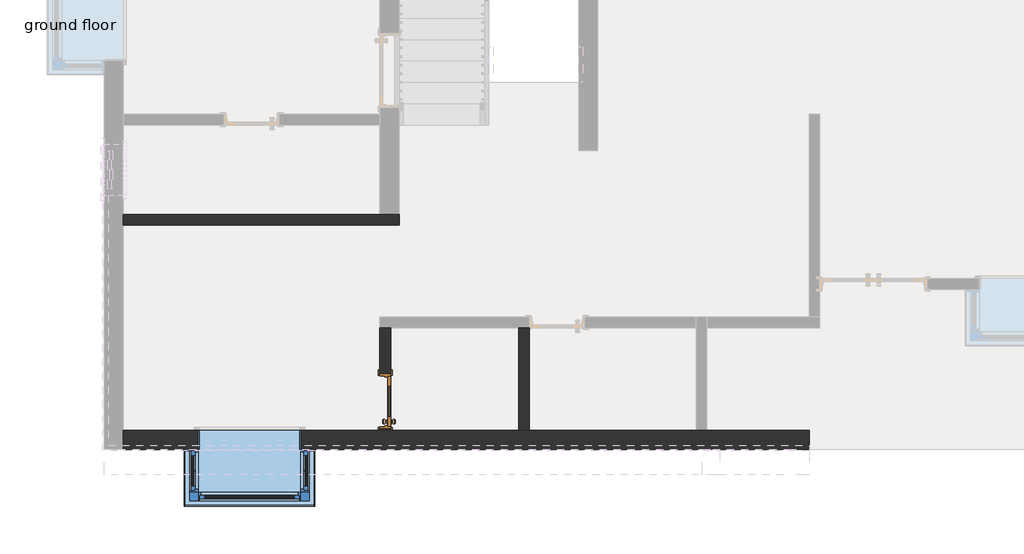
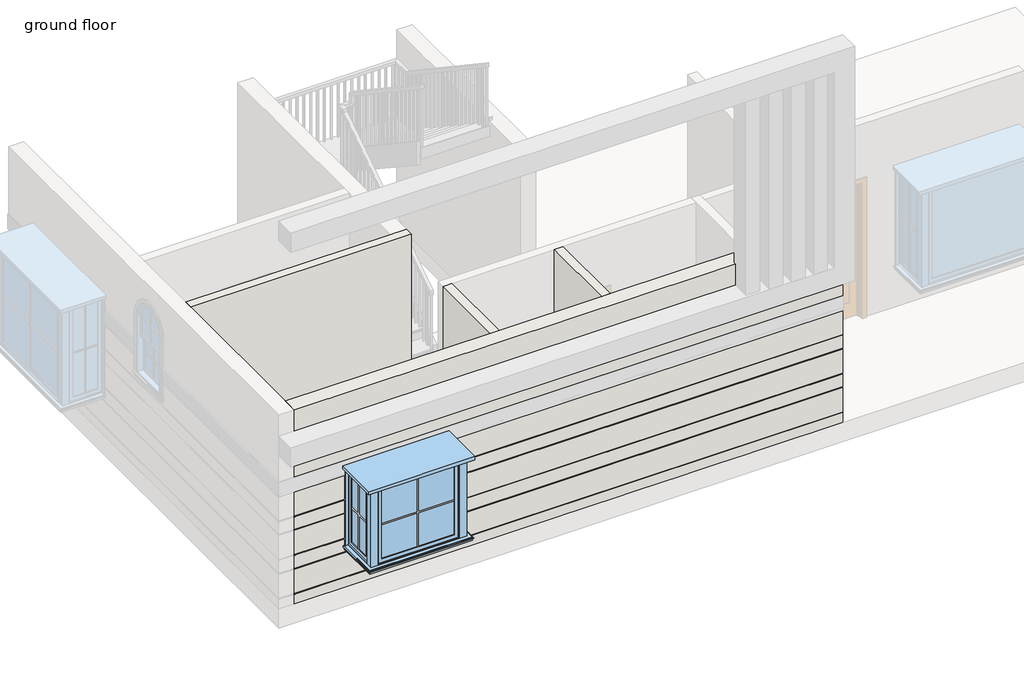
# One storey, part 1 of 5: 4 walls, 1 door, 1 window.
"""IFC4 building model written with IfcOpenShell, lengths in millimetres."""

from ifc_helpers import new_model, si_unit, frame, origin, place, context, project, spatial, polyline, circle_curve, outline, extrude, faceted_brep, transform, mapped, element, save
from ifc_brep_helpers import plane_surface, cylinder_surface, revolved_surface, advanced_brep
from components import door_e337afa5, window_4fde904e

model = new_model("IFC4")

# Units and contexts
model_context = context("Model", 3, world=origin())
ifc_project = project(units=[si_unit("LENGTHUNIT", "METRE", prefix="MILLI")], contexts=[model_context])

# Site, building, storey
site = spatial("IfcSite", under=ifc_project)
building = spatial("IfcBuilding", under=site)
storey = spatial("IfcBuildingStorey", under=building, Name="ground floor", Elevation=304.8)

# Door
placement = place(None, origin())
door_shape = door_e337afa5(model_context)
element("IfcDoor", 1, ObjectType="Door-Interior-Single-2_Panel-Wood : 24\" x 84\"", at=placement, inside=storey, context=model_context, shape_type="MappedRepresentation", body=[
    mapped(door_shape, transform((-9835.7922301, -6693.7302427, 304.8), x_axis=(0.0, 1.0, 0.0), y_axis=(-1.0, 0.0, 0.0), z_axis=(0.0, 0.0, 1.0))),
])

# Walls
element("IfcWall", 2, ObjectType="INNER WALL 5\"", at=placement, inside=storey, context=model_context, shape_type="Brep", body=[
    faceted_brep([(-12950.4672301, -4598.2302427, 304.8), (-9673.8672301, -4598.2302427, 304.8), (-9673.8672301, -4598.2302427, 3352.8), (-12950.4672301, -4598.2302427, 3352.8), (-12950.4672301, -4471.2302427, 304.8), (-12950.4672301, -4471.2302427, 3352.8), (-9902.4672301, -4471.2302427, 3352.8), (-9673.8672301, -4471.2302427, 3352.8), (-9673.8672301, -4471.2302427, 304.8), (-9902.4672301, -4471.2302427, 304.8)], [[[0, 1, 2, 3]], [[4, 5, 6, 7, 8, 9]], [[1, 0, 4, 9, 8]], [[3, 2, 7, 6, 5]], [[0, 3, 5, 4]], [[2, 1, 8, 7]]]),
])
element("IfcWall", 3, ObjectType="INNER WALL 5\"", at=placement, inside=storey, context=model_context, shape_type="Brep", body=[
    faceted_brep([(-8124.4672301, -7036.6302427, 304.8), (-8124.4672301, -5817.4302427, 304.8), (-8124.4672301, -5817.4302427, 2463.8), (-8124.4672301, -5817.4302427, 3352.8), (-8124.4672301, -7036.6302427, 3352.8), (-8251.4672301, -7036.6302427, 304.8), (-8251.4672301, -7036.6302427, 3352.8), (-8251.4672301, -5817.4302427, 3352.8), (-8251.4672301, -5817.4302427, 304.8)], [[[0, 1, 2, 3, 4]], [[5, 6, 7, 8]], [[1, 0, 5, 8]], [[4, 3, 7, 6]], [[0, 4, 6, 5]], [[3, 2, 1, 8, 7]]]),
])
element("IfcWall", 4, ObjectType="INNER WALL 5\"", at=placement, inside=storey, context=model_context, shape_type="SweptSolid", body=[
    extrude(outline(polyline([(-7036.6302427, 3352.8), (-5817.4302427, 3352.8), (-5817.4302427, 304.8), (-6363.5302427, 304.8), (-6363.5302427, 2463.8), (-7023.9302427, 2463.8), (-7023.9302427, 304.8), (-7036.6302427, 304.8), (-7036.6302427, 3352.8)])), frame((-9902.4672301, 0.0, 0.0), z_axis=(1.0, 0.0, 0.0), x_axis=(0.0, 1.0, 0.0)), (0.0, 0.0, 1.0), 127.0),
])
element("IfcWall", 5, ObjectType="OUTER WALL 9\"", at=placement, inside=storey, context=model_context, shape_type="AdvancedBrep", body=[
    advanced_brep(
    [(-12950.4672301, -7265.2302427, 304.8), (-4797.0672301, -7265.2302427, 304.8), (-4797.0672301, -7265.2302427, 455.95311), (-12950.4672301, -7265.2302427, 455.95311), (-4797.0672301, -7265.2302427, 3352.8), (-12950.4672301, -7265.2302427, 3352.8), (-12950.4672301, -7265.2302427, 2298.7), (-4797.0672301, -7265.2302427, 2298.7), (-10842.2672301, -7265.2302427, 914.4), (-12061.4672301, -7265.2302427, 914.4), (-12061.4672301, -7265.2302427, 1065.55311), (-12950.4672301, -7265.2302427, 1065.55311), (-12950.4672301, -7265.2302427, 864.84689), (-12061.4672301, -7265.2302427, 864.84689), (-12061.4672301, -7265.2302427, 850.9), (-12950.4672301, -7265.2302427, 850.9), (-12950.4672301, -7265.2302427, 469.9), (-4797.0672301, -7265.2302427, 469.9), (-4797.0672301, -7265.2302427, 850.9), (-10842.2672301, -7265.2302427, 850.9), (-10842.2672301, -7265.2302427, 864.84689), (-4797.0672301, -7265.2302427, 864.84689), (-4797.0672301, -7265.2302427, 1065.55311), (-10842.2672301, -7265.2302427, 1065.55311), (-12061.4672301, -7265.2302427, 2184.4), (-10842.2672301, -7265.2302427, 2184.4), (-10842.2672301, -7265.2302427, 2084.04689), (-4797.0672301, -7265.2302427, 2084.04689), (-4797.0672301, -7265.2302427, 2284.75311), (-12950.4672301, -7265.2302427, 2284.75311), (-12950.4672301, -7265.2302427, 2084.04689), (-12061.4672301, -7265.2302427, 2084.04689), (-10842.2672301, -7265.2302427, 2070.1), (-10842.2672301, -7265.2302427, 1689.1), (-4797.0672301, -7265.2302427, 1689.1), (-4797.0672301, -7265.2302427, 2070.1), (-10842.2672301, -7265.2302427, 1675.15311), (-10842.2672301, -7265.2302427, 1474.44689), (-4797.0672301, -7265.2302427, 1474.44689), (-4797.0672301, -7265.2302427, 1675.15311), (-12061.4672301, -7265.2302427, 1474.44689), (-12061.4672301, -7265.2302427, 1675.15311), (-12950.4672301, -7265.2302427, 1675.15311), (-12950.4672301, -7265.2302427, 1474.44689), (-4797.0672301, -7265.2302427, 1460.5), (-10842.2672301, -7265.2302427, 1460.5), (-10842.2672301, -7265.2302427, 1079.5), (-4797.0672301, -7265.2302427, 1079.5), (-12061.4672301, -7265.2302427, 2070.1), (-12950.4672301, -7265.2302427, 2070.1), (-12950.4672301, -7265.2302427, 1689.1), (-12061.4672301, -7265.2302427, 1689.1), (-12061.4672301, -7265.2302427, 1460.5), (-12950.4672301, -7265.2302427, 1460.5), (-12950.4672301, -7265.2302427, 1079.5), (-12061.4672301, -7265.2302427, 1079.5), (-4797.0672301, -7036.6302427, 304.8), (-6016.2672301, -7036.6302427, 304.8), (-6143.2672301, -7036.6302427, 304.8), (-8124.4672301, -7036.6302427, 304.8), (-8251.4672301, -7036.6302427, 304.8), (-9775.4672301, -7036.6302427, 304.8), (-9902.4672301, -7036.6302427, 304.8), (-12950.4672301, -7036.6302427, 304.8), (-12950.4672301, -7036.6302427, 3352.8), (-9902.4672301, -7036.6302427, 3352.8), (-9775.4672301, -7036.6302427, 3352.8), (-8251.4672301, -7036.6302427, 3352.8), (-8124.4672301, -7036.6302427, 3352.8), (-6143.2672301, -7036.6302427, 3352.8), (-6016.2672301, -7036.6302427, 3352.8), (-4797.0672301, -7036.6302427, 3352.8), (-12061.4672301, -7036.6302427, 2184.4), (-12061.4672301, -7036.6302427, 914.4), (-10842.2672301, -7036.6302427, 914.4), (-10842.2672301, -7036.6302427, 2184.4), (-4797.0672301, -7216.8686427, 2298.7), (-4797.0672301, -7216.8686427, 2297.3203242), (-4797.0672301, -7221.2514519, 2292.1465897), (-4797.0672301, -7264.1100243, 2285.00348), (-4797.0672301, -7264.1100243, 2083.79652), (-4797.0672301, -7221.2514519, 2076.6534103), (-4797.0672301, -7216.8686427, 2071.4796758), (-4797.0672301, -7216.8686427, 2070.1), (-4797.0672301, -7216.8686427, 1689.1), (-4797.0672301, -7216.8686427, 1687.7203242), (-4797.0672301, -7221.2514519, 1682.5465897), (-4797.0672301, -7264.1100243, 1675.40348), (-4797.0672301, -7264.1100243, 1474.19652), (-4797.0672301, -7221.2514519, 1467.0534103), (-4797.0672301, -7216.8686427, 1461.8796758), (-4797.0672301, -7216.8686427, 1460.5), (-4797.0672301, -7216.8686427, 1079.5), (-4797.0672301, -7216.8686427, 1078.1203242), (-4797.0672301, -7221.2514519, 1072.9465897), (-4797.0672301, -7264.1100243, 1065.80348), (-4797.0672301, -7264.1100243, 864.59652), (-4797.0672301, -7221.2514519, 857.4534103), (-4797.0672301, -7216.8686427, 852.2796758), (-4797.0672301, -7216.8686427, 850.9), (-4797.0672301, -7216.8686427, 469.9), (-4797.0672301, -7216.8686427, 468.5203242), (-4797.0672301, -7221.2514519, 463.3465897), (-4797.0672301, -7264.1100243, 456.20348), (-12950.4672301, -7264.1100243, 456.20348), (-12950.4672301, -7221.2514519, 463.3465897), (-12950.4672301, -7216.8686427, 468.5203242), (-12950.4672301, -7216.8686427, 469.9), (-12950.4672301, -7216.8686427, 850.9), (-12950.4672301, -7216.8686427, 852.2796758), (-12950.4672301, -7221.2514519, 857.4534103), (-12950.4672301, -7264.1100243, 864.59652), (-12950.4672301, -7264.1100243, 1065.80348), (-12950.4672301, -7221.2514519, 1072.9465897), (-12950.4672301, -7216.8686427, 1078.1203242), (-12950.4672301, -7216.8686427, 1079.5), (-12950.4672301, -7216.8686427, 1460.5), (-12950.4672301, -7216.8686427, 1461.8796758), (-12950.4672301, -7221.2514519, 1467.0534103), (-12950.4672301, -7264.1100243, 1474.19652), (-12950.4672301, -7264.1100243, 1675.40348), (-12950.4672301, -7221.2514519, 1682.5465897), (-12950.4672301, -7216.8686427, 1687.7203242), (-12950.4672301, -7216.8686427, 1689.1), (-12950.4672301, -7216.8686427, 2070.1), (-12950.4672301, -7216.8686427, 2071.4796758), (-12950.4672301, -7221.2514519, 2076.6534103), (-12950.4672301, -7264.1100243, 2083.79652), (-12950.4672301, -7264.1100243, 2285.00348), (-12950.4672301, -7221.2514519, 2292.1465897), (-12950.4672301, -7216.8686427, 2297.3203242), (-12950.4672301, -7216.8686427, 2298.7), (-12061.4672301, -7264.1100243, 2083.79652), (-12061.4672301, -7221.2514519, 2076.6534103), (-12061.4672301, -7216.8686427, 2071.4796758), (-12061.4672301, -7216.8686427, 2070.1), (-12061.4672301, -7216.8686427, 1689.1), (-12061.4672301, -7216.8686427, 1687.7203242), (-12061.4672301, -7221.2514519, 1682.5465897), (-12061.4672301, -7264.1100243, 1675.40348), (-12061.4672301, -7264.1100243, 1474.19652), (-12061.4672301, -7221.2514519, 1467.0534103), (-12061.4672301, -7216.8686427, 1461.8796758), (-12061.4672301, -7216.8686427, 1460.5), (-12061.4672301, -7216.8686427, 1079.5), (-12061.4672301, -7216.8686427, 1078.1203242), (-12061.4672301, -7221.2514519, 1072.9465897), (-12061.4672301, -7264.1100243, 1065.80348), (-10842.2672301, -7264.1100243, 1065.80348), (-10842.2672301, -7221.2514519, 1072.9465897), (-10842.2672301, -7216.8686427, 1078.1203242), (-10842.2672301, -7216.8686427, 1079.5), (-10842.2672301, -7216.8686427, 1460.5), (-10842.2672301, -7216.8686427, 1461.8796758), (-10842.2672301, -7221.2514519, 1467.0534103), (-10842.2672301, -7264.1100243, 1474.19652), (-10842.2672301, -7264.1100243, 1675.40348), (-10842.2672301, -7221.2514519, 1682.5465897), (-10842.2672301, -7216.8686427, 1687.7203242), (-10842.2672301, -7216.8686427, 1689.1), (-10842.2672301, -7216.8686427, 2070.1), (-10842.2672301, -7216.8686427, 2071.4796758), (-10842.2672301, -7221.2514519, 2076.6534103), (-10842.2672301, -7264.1100243, 2083.79652), (-10842.2672301, -7221.2514519, 857.4534103), (-10842.2672301, -7264.1100243, 864.59652), (-10842.2672301, -7216.8686427, 850.9), (-10842.2672301, -7216.8686427, 852.2796758), (-12061.4672301, -7216.8686427, 852.2796758), (-12061.4672301, -7216.8686427, 850.9), (-12061.4672301, -7264.1100243, 864.59652), (-12061.4672301, -7221.2514519, 857.4534103)],
    [
        (0, 1),
        (1, 2),
        (2, 3),
        (3, 0),
        (4, 5),
        (5, 6),
        (6, 7),
        (7, 4),
        (8, 9),
        (9, 10),
        (10, 11),
        (11, 12),
        (12, 13),
        (13, 14),
        (14, 15),
        (15, 16),
        (16, 17),
        (17, 18),
        (18, 19),
        (19, 20),
        (20, 21),
        (21, 22),
        (22, 23),
        (23, 8),
        (24, 25),
        (25, 26),
        (26, 27),
        (27, 28),
        (28, 29),
        (29, 30),
        (30, 31),
        (31, 24),
        (32, 33),
        (33, 34),
        (34, 35),
        (35, 32),
        (36, 37),
        (37, 38),
        (38, 39),
        (39, 36),
        (40, 41),
        (41, 42),
        (42, 43),
        (43, 40),
        (44, 45),
        (45, 46),
        (46, 47),
        (47, 44),
        (48, 49),
        (49, 50),
        (50, 51),
        (51, 48),
        (52, 53),
        (53, 54),
        (54, 55),
        (55, 52),
        (56, 57),
        (57, 58),
        (58, 59),
        (59, 60),
        (60, 61),
        (61, 62),
        (62, 63),
        (63, 64),
        (64, 65),
        (65, 66),
        (66, 67),
        (67, 68),
        (68, 69),
        (69, 70),
        (70, 71),
        (71, 56),
        (72, 73),
        (73, 74),
        (74, 75),
        (75, 72),
        (0, 63),
        (56, 1),
        (71, 4),
        (7, 76),
        (76, 77),
        (77, 78, circle_curve(frame((-4797.0672301, -7222.1137427, 2297.3203242), z_axis=(-1.0, 0.0, 0.0), x_axis=(0.0, 1.0, 0.0)), 5.2451)),
        (78, 79),
        (79, 28, circle_curve(frame((-4797.0672301, -7262.3854427, 2274.656011), z_axis=(1.0, 0.0, 0.0), x_axis=(0.0, 1.0, 0.0)), 10.4902)),
        (27, 80, circle_curve(frame((-4797.0672301, -7262.3854427, 2094.143989), z_axis=(1.0, 0.0, 0.0), x_axis=(0.0, 1.0, 0.0)), 10.4902)),
        (80, 81),
        (81, 82, circle_curve(frame((-4797.0672301, -7222.1137427, 2071.4796758), z_axis=(-1.0, 0.0, 0.0), x_axis=(0.0, 1.0, 0.0)), 5.2451)),
        (82, 83),
        (83, 35),
        (34, 84),
        (84, 85),
        (85, 86, circle_curve(frame((-4797.0672301, -7222.1137427, 1687.7203242), z_axis=(-1.0, 0.0, 0.0), x_axis=(0.0, 1.0, 0.0)), 5.2451)),
        (86, 87),
        (87, 39, circle_curve(frame((-4797.0672301, -7262.3854427, 1665.056011), z_axis=(1.0, 0.0, 0.0), x_axis=(0.0, 1.0, 0.0)), 10.4902)),
        (38, 88, circle_curve(frame((-4797.0672301, -7262.3854427, 1484.543989), z_axis=(1.0, 0.0, 0.0), x_axis=(0.0, 1.0, 0.0)), 10.4902)),
        (88, 89),
        (89, 90, circle_curve(frame((-4797.0672301, -7222.1137427, 1461.8796758), z_axis=(-1.0, 0.0, 0.0), x_axis=(0.0, 1.0, 0.0)), 5.2451)),
        (90, 91),
        (91, 44),
        (47, 92),
        (92, 93),
        (93, 94, circle_curve(frame((-4797.0672301, -7222.1137427, 1078.1203242), z_axis=(-1.0, 0.0, 0.0), x_axis=(0.0, 1.0, 0.0)), 5.2451)),
        (94, 95),
        (95, 22, circle_curve(frame((-4797.0672301, -7262.3854427, 1055.456011), z_axis=(1.0, 0.0, 0.0), x_axis=(0.0, 1.0, 0.0)), 10.4902)),
        (21, 96, circle_curve(frame((-4797.0672301, -7262.3854427, 874.943989), z_axis=(1.0, 0.0, 0.0), x_axis=(0.0, 1.0, 0.0)), 10.4902)),
        (96, 97),
        (97, 98, circle_curve(frame((-4797.0672301, -7222.1137427, 852.2796758), z_axis=(-1.0, 0.0, 0.0), x_axis=(0.0, 1.0, 0.0)), 5.2451)),
        (98, 99),
        (99, 18),
        (17, 100),
        (100, 101),
        (101, 102, circle_curve(frame((-4797.0672301, -7222.1137427, 468.5203242), z_axis=(-1.0, 0.0, 0.0), x_axis=(0.0, 1.0, 0.0)), 5.2451)),
        (102, 103),
        (103, 2, circle_curve(frame((-4797.0672301, -7262.3854427, 445.856011), z_axis=(1.0, 0.0, 0.0), x_axis=(0.0, 1.0, 0.0)), 10.4902)),
        (64, 5),
        (3, 104, circle_curve(frame((-12950.4672301, -7262.3854427, 445.856011), z_axis=(-1.0, 0.0, 0.0), x_axis=(0.0, 1.0, 0.0)), 10.4902)),
        (104, 105),
        (105, 106, circle_curve(frame((-12950.4672301, -7222.1137427, 468.5203242), z_axis=(1.0, 0.0, 0.0), x_axis=(0.0, 1.0, 0.0)), 5.2451)),
        (106, 107),
        (107, 16),
        (15, 108),
        (108, 109),
        (109, 110, circle_curve(frame((-12950.4672301, -7222.1137427, 852.2796758), z_axis=(1.0, 0.0, 0.0), x_axis=(0.0, 1.0, 0.0)), 5.2451)),
        (110, 111),
        (111, 12, circle_curve(frame((-12950.4672301, -7262.3854427, 874.943989), z_axis=(-1.0, 0.0, 0.0), x_axis=(0.0, 1.0, 0.0)), 10.4902)),
        (11, 112, circle_curve(frame((-12950.4672301, -7262.3854427, 1055.456011), z_axis=(-1.0, 0.0, 0.0), x_axis=(0.0, 1.0, 0.0)), 10.4902)),
        (112, 113),
        (113, 114, circle_curve(frame((-12950.4672301, -7222.1137427, 1078.1203242), z_axis=(1.0, 0.0, 0.0), x_axis=(0.0, 1.0, 0.0)), 5.2451)),
        (114, 115),
        (115, 54),
        (53, 116),
        (116, 117),
        (117, 118, circle_curve(frame((-12950.4672301, -7222.1137427, 1461.8796758), z_axis=(1.0, 0.0, 0.0), x_axis=(0.0, 1.0, 0.0)), 5.2451)),
        (118, 119),
        (119, 43, circle_curve(frame((-12950.4672301, -7262.3854427, 1484.543989), z_axis=(-1.0, 0.0, 0.0), x_axis=(0.0, 1.0, 0.0)), 10.4902)),
        (42, 120, circle_curve(frame((-12950.4672301, -7262.3854427, 1665.056011), z_axis=(-1.0, 0.0, 0.0), x_axis=(0.0, 1.0, 0.0)), 10.4902)),
        (120, 121),
        (121, 122, circle_curve(frame((-12950.4672301, -7222.1137427, 1687.7203242), z_axis=(1.0, 0.0, 0.0), x_axis=(0.0, 1.0, 0.0)), 5.2451)),
        (122, 123),
        (123, 50),
        (49, 124),
        (124, 125),
        (125, 126, circle_curve(frame((-12950.4672301, -7222.1137427, 2071.4796758), z_axis=(1.0, 0.0, 0.0), x_axis=(0.0, 1.0, 0.0)), 5.2451)),
        (126, 127),
        (127, 30, circle_curve(frame((-12950.4672301, -7262.3854427, 2094.143989), z_axis=(-1.0, 0.0, 0.0), x_axis=(0.0, 1.0, 0.0)), 10.4902)),
        (29, 128, circle_curve(frame((-12950.4672301, -7262.3854427, 2274.656011), z_axis=(-1.0, 0.0, 0.0), x_axis=(0.0, 1.0, 0.0)), 10.4902)),
        (128, 129),
        (129, 130, circle_curve(frame((-12950.4672301, -7222.1137427, 2297.3203242), z_axis=(1.0, 0.0, 0.0), x_axis=(0.0, 1.0, 0.0)), 5.2451)),
        (130, 131),
        (131, 6),
        (72, 24),
        (31, 132, circle_curve(frame((-12061.4672301, -7262.3854427, 2094.143989), z_axis=(1.0, 0.0, 0.0), x_axis=(0.0, 1.0, 0.0)), 10.4902)),
        (132, 133),
        (133, 134, circle_curve(frame((-12061.4672301, -7222.1137427, 2071.4796758), z_axis=(-1.0, 0.0, 0.0), x_axis=(0.0, 1.0, 0.0)), 5.2451)),
        (134, 135),
        (135, 48),
        (51, 136),
        (136, 137),
        (137, 138, circle_curve(frame((-12061.4672301, -7222.1137427, 1687.7203242), z_axis=(-1.0, 0.0, 0.0), x_axis=(0.0, 1.0, 0.0)), 5.2451)),
        (138, 139),
        (139, 41, circle_curve(frame((-12061.4672301, -7262.3854427, 1665.056011), z_axis=(1.0, 0.0, 0.0), x_axis=(0.0, 1.0, 0.0)), 10.4902)),
        (40, 140, circle_curve(frame((-12061.4672301, -7262.3854427, 1484.543989), z_axis=(1.0, 0.0, 0.0), x_axis=(0.0, 1.0, 0.0)), 10.4902)),
        (140, 141),
        (141, 142, circle_curve(frame((-12061.4672301, -7222.1137427, 1461.8796758), z_axis=(-1.0, 0.0, 0.0), x_axis=(0.0, 1.0, 0.0)), 5.2451)),
        (142, 143),
        (143, 52),
        (55, 144),
        (144, 145),
        (145, 146, circle_curve(frame((-12061.4672301, -7222.1137427, 1078.1203242), z_axis=(-1.0, 0.0, 0.0), x_axis=(0.0, 1.0, 0.0)), 5.2451)),
        (146, 147),
        (147, 10, circle_curve(frame((-12061.4672301, -7262.3854427, 1055.456011), z_axis=(1.0, 0.0, 0.0), x_axis=(0.0, 1.0, 0.0)), 10.4902)),
        (9, 73),
        (8, 74),
        (23, 148, circle_curve(frame((-10842.2672301, -7262.3854427, 1055.456011), z_axis=(-1.0, 0.0, 0.0), x_axis=(0.0, 1.0, 0.0)), 10.4902)),
        (148, 149),
        (149, 150, circle_curve(frame((-10842.2672301, -7222.1137427, 1078.1203242), z_axis=(1.0, 0.0, 0.0), x_axis=(0.0, 1.0, 0.0)), 5.2451)),
        (150, 151),
        (151, 46),
        (45, 152),
        (152, 153),
        (153, 154, circle_curve(frame((-10842.2672301, -7222.1137427, 1461.8796758), z_axis=(1.0, 0.0, 0.0), x_axis=(0.0, 1.0, 0.0)), 5.2451)),
        (154, 155),
        (155, 37, circle_curve(frame((-10842.2672301, -7262.3854427, 1484.543989), z_axis=(-1.0, 0.0, 0.0), x_axis=(0.0, 1.0, 0.0)), 10.4902)),
        (36, 156, circle_curve(frame((-10842.2672301, -7262.3854427, 1665.056011), z_axis=(-1.0, 0.0, 0.0), x_axis=(0.0, 1.0, 0.0)), 10.4902)),
        (156, 157),
        (157, 158, circle_curve(frame((-10842.2672301, -7222.1137427, 1687.7203242), z_axis=(1.0, 0.0, 0.0), x_axis=(0.0, 1.0, 0.0)), 5.2451)),
        (158, 159),
        (159, 33),
        (32, 160),
        (160, 161),
        (161, 162, circle_curve(frame((-10842.2672301, -7222.1137427, 2071.4796758), z_axis=(1.0, 0.0, 0.0), x_axis=(0.0, 1.0, 0.0)), 5.2451)),
        (162, 163),
        (163, 26, circle_curve(frame((-10842.2672301, -7262.3854427, 2094.143989), z_axis=(-1.0, 0.0, 0.0), x_axis=(0.0, 1.0, 0.0)), 10.4902)),
        (25, 75),
        (76, 131),
        (130, 77),
        (129, 78),
        (128, 79),
        (127, 132),
        (163, 80),
        (126, 133),
        (162, 81),
        (125, 134),
        (161, 82),
        (124, 135),
        (160, 83),
        (159, 84),
        (158, 85),
        (157, 86),
        (156, 87),
        (155, 88),
        (154, 89),
        (153, 90),
        (152, 91),
        (136, 123),
        (122, 137),
        (121, 138),
        (120, 139),
        (119, 140),
        (118, 141),
        (117, 142),
        (116, 143),
        (164, 165),
        (165, 20, circle_curve(frame((-10842.2672301, -7262.3854427, 874.943989), z_axis=(-1.0, 0.0, 0.0), x_axis=(0.0, 1.0, 0.0)), 10.4902)),
        (19, 166),
        (166, 167),
        (167, 164, circle_curve(frame((-10842.2672301, -7222.1137427, 852.2796758), z_axis=(1.0, 0.0, 0.0), x_axis=(0.0, 1.0, 0.0)), 5.2451)),
        (151, 92),
        (150, 93),
        (149, 94),
        (148, 95),
        (165, 96),
        (164, 97),
        (167, 98),
        (166, 99),
        (168, 169),
        (169, 14),
        (13, 170, circle_curve(frame((-12061.4672301, -7262.3854427, 874.943989), z_axis=(1.0, 0.0, 0.0), x_axis=(0.0, 1.0, 0.0)), 10.4902)),
        (170, 171),
        (171, 168, circle_curve(frame((-12061.4672301, -7222.1137427, 852.2796758), z_axis=(-1.0, 0.0, 0.0), x_axis=(0.0, 1.0, 0.0)), 5.2451)),
        (144, 115),
        (114, 145),
        (113, 146),
        (112, 147),
        (111, 170),
        (110, 171),
        (109, 168),
        (108, 169),
        (100, 107),
        (106, 101),
        (105, 102),
        (104, 103),
    ],
    [
        plane_surface(frame((-13179.0672301, -7265.2302427, 304.8), z_axis=(0.0, -1.0, 0.0), x_axis=(1.0, 0.0, 0.0))),
        plane_surface(frame((-13179.0672301, -7036.6302427, 304.8), z_axis=(0.0, 1.0, 0.0), x_axis=(-1.0, 0.0, 0.0))),
        plane_surface(frame((-13064.7672301, -7265.2302427, 304.8), z_axis=(0.0, 0.0, -1.0), x_axis=(0.0, 1.0, 0.0))),
        plane_surface(frame((-4797.0672301, -7265.2302427, 304.8), z_axis=(1.0, 0.0, 0.0), x_axis=(0.0, 1.0, 0.0))),
        plane_surface(frame((-4797.0672301, -7265.2302427, 3352.8), z_axis=(0.0, 0.0, 1.0), x_axis=(0.0, 1.0, 0.0))),
        plane_surface(frame((-12950.4672301, -305.6302427, 304.8), z_axis=(-1.0, 0.0, 0.0), x_axis=(0.0, 1.0, 0.0))),
        plane_surface(frame((-12061.4672301, -7036.6302427, 2184.4), z_axis=(1.0, 0.0, 0.0), x_axis=(0.0, -1.0, 0.0))),
        plane_surface(frame((-12061.4672301, -7036.6302427, 914.4), z_axis=(0.0, 0.0, 1.0), x_axis=(0.0, -1.0, 0.0))),
        plane_surface(frame((-10842.2672301, -7036.6302427, 914.4), z_axis=(-1.0, 0.0, 0.0), x_axis=(0.0, -1.0, 0.0))),
        plane_surface(frame((-10842.2672301, -7036.6302427, 2184.4), z_axis=(0.0, 0.0, -1.0), x_axis=(0.0, -1.0, 0.0))),
        plane_surface(frame((-13130.7056301, -7216.8686427, 2298.7), z_axis=(0.0, -1.0, 0.0), x_axis=(1.0, 0.0, 0.0))),
        revolved_surface(polyline([(-12950.4672301, -7216.8686427, 2297.3203242), (-4797.0672300999995, -7216.8686427, 2297.3203242)]), (-13179.0672301, -7222.1137427, 2297.3203242), (-1.0, 0.0, 0.0)),
        plane_surface(frame((-13158.7091301, -7244.8721427, 2288.2098), z_axis=(0.0, -0.16439930721687152, 0.9863938705135048), x_axis=(1.0, 0.0, 0.0))),
        cylinder_surface(frame((-13179.0672301, -7262.3854427, 2274.656011), z_axis=(1.0, 0.0, 0.0), x_axis=(0.0, 1.0, 0.0)), 10.4902),
        cylinder_surface(frame((-13179.0672301, -7262.3854427, 2094.143989), z_axis=(1.0, 0.0, 0.0), x_axis=(0.0, 1.0, 0.0)), 10.4902),
        plane_surface(frame((-13158.7091301, -7244.8721427, 2080.5902), z_axis=(0.0, -0.16439930721687798, -0.9863938705135037), x_axis=(1.0, 0.0, 0.0))),
        revolved_surface(polyline([(-12950.4672301, -7216.8686427, 2071.4796758), (-12061.4672301, -7216.8686427, 2071.4796758)]), (-13179.0672301, -7222.1137427, 2071.4796758), (-1.0, 0.0, 0.0)),
        revolved_surface(polyline([(-10842.2672301, -7216.8686427, 2071.4796758), (-4797.0672300999995, -7216.8686427, 2071.4796758)]), (-13179.0672301, -7222.1137427, 2071.4796758), (-1.0, 0.0, 0.0)),
        plane_surface(frame((-13130.7056301, -7216.8686427, 2071.4796758), z_axis=(0.0, -1.0, 0.0), x_axis=(1.0, 0.0, 0.0))),
        plane_surface(frame((-10842.2672301, -7280.1146427, 1689.1), z_axis=(0.0, 0.0, -1.0), x_axis=(1.0, 0.0, 0.0))),
        plane_surface(frame((-10842.2672301, -7216.8686427, 1689.1), z_axis=(0.0, -1.0, 0.0), x_axis=(1.0, 0.0, 0.0))),
        revolved_surface(polyline([(-10842.2672301, -7216.8686427, 1687.7203242), (-4797.0672301, -7216.8686427, 1687.7203242)]), (-10842.2672301, -7222.1137427, 1687.7203242), (-1.0, 0.0, 0.0)),
        plane_surface(frame((-10842.2672301, -7244.8721427, 1678.6098), z_axis=(0.0, -0.16439930721687146, 0.9863938705135048), x_axis=(1.0, 0.0, 0.0))),
        cylinder_surface(frame((-10842.2672301, -7262.3854427, 1665.056011), z_axis=(1.0, 0.0, 0.0), x_axis=(0.0, 1.0, 0.0)), 10.4902),
        cylinder_surface(frame((-10842.2672301, -7262.3854427, 1484.543989), z_axis=(1.0, 0.0, 0.0), x_axis=(0.0, 1.0, 0.0)), 10.4902),
        plane_surface(frame((-10842.2672301, -7244.8721427, 1470.9902), z_axis=(0.0, -0.16439930721687793, -0.9863938705135037), x_axis=(1.0, 0.0, 0.0))),
        revolved_surface(polyline([(-10842.2672301, -7216.8686427, 1461.8796758), (-4797.0672301, -7216.8686427, 1461.8796758)]), (-10842.2672301, -7222.1137427, 1461.8796758), (-1.0, 0.0, 0.0)),
        plane_surface(frame((-10842.2672301, -7216.8686427, 1461.8796758), z_axis=(0.0, -1.0, 0.0), x_axis=(1.0, 0.0, 0.0))),
        plane_surface(frame((-10842.2672301, -7216.8686427, 1460.5), z_axis=(0.0, 0.0, 1.0), x_axis=(1.0, 0.0, 0.0))),
        plane_surface(frame((-13130.7056301, -7216.8686427, 1689.1), z_axis=(0.0, -1.0, 0.0), x_axis=(1.0, 0.0, 0.0))),
        revolved_surface(polyline([(-12950.4672301, -7216.8686427, 1687.7203242), (-12061.4672301, -7216.8686427, 1687.7203242)]), (-13179.0672301, -7222.1137427, 1687.7203242), (-1.0, 0.0, 0.0)),
        plane_surface(frame((-13158.7091301, -7244.8721427, 1678.6098), z_axis=(0.0, -0.16439930721687152, 0.9863938705135048), x_axis=(1.0, 0.0, 0.0))),
        cylinder_surface(frame((-13179.0672301, -7262.3854427, 1665.056011), z_axis=(1.0, 0.0, 0.0), x_axis=(0.0, 1.0, 0.0)), 10.4902),
        cylinder_surface(frame((-13179.0672301, -7262.3854427, 1484.543989), z_axis=(1.0, 0.0, 0.0), x_axis=(0.0, 1.0, 0.0)), 10.4902),
        plane_surface(frame((-13158.7091301, -7244.8721427, 1470.9902), z_axis=(0.0, -0.16439930721687798, -0.9863938705135037), x_axis=(1.0, 0.0, 0.0))),
        revolved_surface(polyline([(-12950.4672301, -7216.8686427, 1461.8796758), (-12061.4672301, -7216.8686427, 1461.8796758)]), (-13179.0672301, -7222.1137427, 1461.8796758), (-1.0, 0.0, 0.0)),
        plane_surface(frame((-13130.7056301, -7216.8686427, 1461.8796758), z_axis=(0.0, -1.0, 0.0), x_axis=(1.0, 0.0, 0.0))),
        plane_surface(frame((-10842.2672301, -7036.6302427, 914.4), z_axis=(1.0, 0.0, 0.0), x_axis=(0.0, -1.0, 0.0))),
        plane_surface(frame((-10842.2672301, -7280.1146427, 1079.5), z_axis=(0.0, 0.0, -1.0), x_axis=(1.0, 0.0, 0.0))),
        plane_surface(frame((-10842.2672301, -7216.8686427, 1079.5), z_axis=(0.0, -1.0, 0.0), x_axis=(1.0, 0.0, 0.0))),
        revolved_surface(polyline([(-10842.2672301, -7216.8686427, 1078.1203242), (-4797.0672301, -7216.8686427, 1078.1203242)]), (-10842.2672301, -7222.1137427, 1078.1203242), (-1.0, 0.0, 0.0)),
        plane_surface(frame((-10842.2672301, -7244.8721427, 1069.0098), z_axis=(0.0, -0.16439930721687146, 0.9863938705135048), x_axis=(1.0, 0.0, 0.0))),
        cylinder_surface(frame((-10842.2672301, -7262.3854427, 1055.456011), z_axis=(1.0, 0.0, 0.0), x_axis=(0.0, 1.0, 0.0)), 10.4902),
        cylinder_surface(frame((-10842.2672301, -7262.3854427, 874.943989), z_axis=(1.0, 0.0, 0.0), x_axis=(0.0, 1.0, 0.0)), 10.4902),
        plane_surface(frame((-10842.2672301, -7244.8721427, 861.3902), z_axis=(0.0, -0.16439930721687793, -0.9863938705135037), x_axis=(1.0, 0.0, 0.0))),
        revolved_surface(polyline([(-10842.2672301, -7216.8686427, 852.2796758), (-4797.0672301, -7216.8686427, 852.2796758)]), (-10842.2672301, -7222.1137427, 852.2796758), (-1.0, 0.0, 0.0)),
        plane_surface(frame((-10842.2672301, -7216.8686427, 852.2796758), z_axis=(0.0, -1.0, 0.0), x_axis=(1.0, 0.0, 0.0))),
        plane_surface(frame((-10842.2672301, -7216.8686427, 850.9), z_axis=(0.0, 0.0, 1.0), x_axis=(1.0, 0.0, 0.0))),
        plane_surface(frame((-12061.4672301, -7036.6302427, 2184.4), z_axis=(-1.0, 0.0, 0.0), x_axis=(0.0, -1.0, 0.0))),
        plane_surface(frame((-13130.7056301, -7216.8686427, 1079.5), z_axis=(0.0, -1.0, 0.0), x_axis=(1.0, 0.0, 0.0))),
        revolved_surface(polyline([(-12950.4672301, -7216.8686427, 1078.1203242), (-12061.4672301, -7216.8686427, 1078.1203242)]), (-13179.0672301, -7222.1137427, 1078.1203242), (-1.0, 0.0, 0.0)),
        plane_surface(frame((-13158.7091301, -7244.8721427, 1069.0098), z_axis=(0.0, -0.16439930721687152, 0.9863938705135048), x_axis=(1.0, 0.0, 0.0))),
        cylinder_surface(frame((-13179.0672301, -7262.3854427, 1055.456011), z_axis=(1.0, 0.0, 0.0), x_axis=(0.0, 1.0, 0.0)), 10.4902),
        cylinder_surface(frame((-13179.0672301, -7262.3854427, 874.943989), z_axis=(1.0, 0.0, 0.0), x_axis=(0.0, 1.0, 0.0)), 10.4902),
        plane_surface(frame((-13158.7091301, -7244.8721427, 861.3902), z_axis=(0.0, -0.16439930721687798, -0.9863938705135037), x_axis=(1.0, 0.0, 0.0))),
        revolved_surface(polyline([(-12950.4672301, -7216.8686427, 852.2796758), (-12061.4672301, -7216.8686427, 852.2796758)]), (-13179.0672301, -7222.1137427, 852.2796758), (-1.0, 0.0, 0.0)),
        plane_surface(frame((-13130.7056301, -7216.8686427, 852.2796758), z_axis=(0.0, -1.0, 0.0), x_axis=(1.0, 0.0, 0.0))),
        plane_surface(frame((-13130.7056301, -7216.8686427, 469.9), z_axis=(0.0, -1.0, 0.0), x_axis=(1.0, 0.0, 0.0))),
        revolved_surface(polyline([(-12950.4672301, -7216.8686427, 468.5203242), (-4797.0672300999995, -7216.8686427, 468.5203242)]), (-13179.0672301, -7222.1137427, 468.5203242), (-1.0, 0.0, 0.0)),
        plane_surface(frame((-13158.7091301, -7244.8721427, 459.4098), z_axis=(0.0, -0.16439930721687146, 0.9863938705135048), x_axis=(1.0, 0.0, 0.0))),
        cylinder_surface(frame((-13179.0672301, -7262.3854427, 445.856011), z_axis=(1.0, 0.0, 0.0), x_axis=(0.0, 1.0, 0.0)), 10.4902),
        plane_surface(frame((-13193.9516301, -4242.6302427, 2298.7), z_axis=(0.0, 0.0, -1.0), x_axis=(0.0, -1.0, 0.0))),
        plane_surface(frame((-13130.7056301, -4242.6302427, 2070.1), z_axis=(0.0, 0.0, 1.0), x_axis=(0.0, -1.0, 0.0))),
        plane_surface(frame((-13193.9516301, -2642.4302427, 1689.1), z_axis=(0.0, 0.0, -1.0), x_axis=(0.0, -1.0, 0.0))),
        plane_surface(frame((-13130.7056301, -2642.4302427, 1460.5), z_axis=(0.0, 0.0, 1.0), x_axis=(0.0, -1.0, 0.0))),
        plane_surface(frame((-13193.9516301, -2642.4302427, 1079.5), z_axis=(0.0, 0.0, -1.0), x_axis=(0.0, -1.0, 0.0))),
        plane_surface(frame((-13130.7056301, -2642.4302427, 850.9), z_axis=(0.0, 0.0, 1.0), x_axis=(0.0, -1.0, 0.0))),
        plane_surface(frame((-13193.9516301, -305.6302427, 469.9), z_axis=(0.0, 0.0, -1.0), x_axis=(0.0, -1.0, 0.0))),
    ],
    [
        (0, [[1, 2, 3, 4]]),
        (0, [[5, 6, 7, 8]]),
        (0, [[9, 10, 11, 12, 13, 14, 15, 16, 17, 18, 19, 20, 21, 22, 23, 24]]),
        (0, [[25, 26, 27, 28, 29, 30, 31, 32]]),
        (0, [[33, 34, 35, 36]]),
        (0, [[37, 38, 39, 40]]),
        (0, [[41, 42, 43, 44]]),
        (0, [[45, 46, 47, 48]]),
        (0, [[49, 50, 51, 52]]),
        (0, [[53, 54, 55, 56]]),
        (1, [[57, 58, 59, 60, 61, 62, 63, 64, 65, 66, 67, 68, 69, 70, 71, 72], [73, 74, 75, 76]]),
        (2, [[-1, 77, -63, -62, -61, -60, -59, -58, -57, 78]]),
        (3, [[-72, 79, -8, 80, 81, 82, 83, 84, -28, 85, 86, 87, 88, 89, -35, 90, 91, 92, 93, 94, -39, 95, 96, 97, 98, 99, -48, 100, 101, 102, 103, 104, -22, 105, 106, 107, 108, 109, -18, 110, 111, 112, 113, 114, -2, -78]]),
        (4, [[-5, -79, -71, -70, -69, -68, -67, -66, -65, 115]]),
        (5, [[-115, -64, -77, -4, 116, 117, 118, 119, 120, -16, 121, 122, 123, 124, 125, -12, 126, 127, 128, 129, 130, -54, 131, 132, 133, 134, 135, -43, 136, 137, 138, 139, 140, -50, 141, 142, 143, 144, 145, -30, 146, 147, 148, 149, 150, -6]]),
        (6, [[-73, 151, -32, 152, 153, 154, 155, 156, -52, 157, 158, 159, 160, 161, -41, 162, 163, 164, 165, 166, -56, 167, 168, 169, 170, 171, -10, 172]]),
        (7, [[-74, -172, -9, 173]]),
        (8, [[-75, -173, -24, 174, 175, 176, 177, 178, -46, 179, 180, 181, 182, 183, -37, 184, 185, 186, 187, 188, -33, 189, 190, 191, 192, 193, -26, 194]]),
        (9, [[-76, -194, -25, -151]]),
        (10, [[195, -149, 196, -81]]),
        (11, [[-196, -148, 197, -82]]),
        (12, [[-197, -147, 198, -83]]),
        (13, [[-198, -146, -29, -84]]),
        (14, [[199, -152, -31, -145]]),
        (14, [[200, -85, -27, -193]]),
        (15, [[-199, -144, 201, -153]]),
        (15, [[-200, -192, 202, -86]]),
        (16, [[-201, -143, 203, -154]]),
        (17, [[-202, -191, 204, -87]]),
        (18, [[-203, -142, 205, -155]]),
        (18, [[-204, -190, 206, -88]]),
        (19, [[207, -90, -34, -188]]),
        (20, [[-207, -187, 208, -91]]),
        (21, [[-208, -186, 209, -92]]),
        (22, [[-209, -185, 210, -93]]),
        (23, [[-210, -184, -40, -94]]),
        (24, [[211, -95, -38, -183]]),
        (25, [[-211, -182, 212, -96]]),
        (26, [[-212, -181, 213, -97]]),
        (27, [[-213, -180, 214, -98]]),
        (28, [[-214, -179, -45, -99]]),
        (29, [[215, -139, 216, -158]]),
        (30, [[-216, -138, 217, -159]]),
        (31, [[-217, -137, 218, -160]]),
        (32, [[-218, -136, -42, -161]]),
        (33, [[219, -162, -44, -135]]),
        (34, [[-219, -134, 220, -163]]),
        (35, [[-220, -133, 221, -164]]),
        (36, [[-221, -132, 222, -165]]),
        (37, [[223, 224, -20, 225, 226, 227]]),
        (38, [[228, -100, -47, -178]]),
        (39, [[-228, -177, 229, -101]]),
        (40, [[-229, -176, 230, -102]]),
        (41, [[-230, -175, 231, -103]]),
        (42, [[-231, -174, -23, -104]]),
        (43, [[232, -105, -21, -224]]),
        (44, [[-223, 233, -106, -232]]),
        (45, [[-227, 234, -107, -233]]),
        (46, [[-226, 235, -108, -234]]),
        (47, [[-235, -225, -19, -109]]),
        (48, [[236, 237, -14, 238, 239, 240]]),
        (49, [[241, -129, 242, -168]]),
        (50, [[-242, -128, 243, -169]]),
        (51, [[-243, -127, 244, -170]]),
        (52, [[-244, -126, -11, -171]]),
        (53, [[-238, -13, -125, 245]]),
        (54, [[-239, -245, -124, 246]]),
        (55, [[-240, -246, -123, 247]]),
        (56, [[-236, -247, -122, 248]]),
        (57, [[249, -119, 250, -111]]),
        (58, [[-250, -118, 251, -112]]),
        (59, [[-251, -117, 252, -113]]),
        (60, [[-252, -116, -3, -114]]),
        (61, [[-195, -80, -7, -150]]),
        (62, [[-205, -141, -49, -156]]),
        (62, [[-206, -189, -36, -89]]),
        (63, [[-215, -157, -51, -140]]),
        (64, [[-222, -131, -53, -166]]),
        (65, [[-241, -167, -55, -130]]),
        (66, [[-237, -248, -121, -15]]),
        (67, [[-249, -110, -17, -120]]),
    ],
),
])

# Window
window_shape = window_4fde904e(model_context)
element("IfcWindow", 6, ObjectType="Window-Bay-Casement-Box-90_Degree_Angle-Center_Fixed : 48\" x 48\" x 24\" 2", at=placement, inside=storey, context=model_context, shape_type="MappedRepresentation", body=[
    mapped(window_shape, transform((-11451.8672301, -7150.9302427, 304.8), x_axis=(-1.0, 0.0, 0.0), y_axis=(0.0, -1.0, 0.0), z_axis=(0.0, 0.0, 1.0))),
])

save(model, "model.ifc")

# Revit data of these elements
# Type "Door-Interior-Single-2_Panel-Wood : 24\" x 84\""
#   Type Mark = "10"
#   Assembly Code = "C1020300"
#   Analytic Construction = "Wooden"
#   Top Rail = 0' - 4 11/16"
#   Thickness = 0' - 1 3/8"
#   Thermal Resistance (R) = 2.5876 (h·ft²·°F)/BTU
#   Swing Angle [instance default] = 90.00°
#   Stiles = 0' - 4 3/4"
#   Rough Width = 2' - 2"
#   Rough Height = 7' - 1"
#   Lock Rail = 0' - 7 1/2"
#   Height = 7' - 0"
#   Width = 2' - 0"
#   Heat Transfer Coefficient (U) = 0.3865 BTU/(h·ft²·°F)
#   Bottom Rail = 0' - 9 1/8"
#   Trim Material = Cherry
#   Panel Material = Cherry
#   Frame Material = Cherry
#   Door Handle Material = Aluminum
#   Visual Light Transmittance = 0
#   Solar Heat Gain Coefficient = 0
#   Wall Closure = (empty or 0)
#   Function = (empty or 0)
# Type "INNER WALL 5\""
#   Assembly Code = "B2010"
#   Layers, outside or top first: 0' - 5" "WARM BEIGE COLOUR" (function 1)
# Type "OUTER WALL 9\""
#   Assembly Code = "B2010"
#   Layers, outside or top first: 0' - 9" "WARM BEIGE COLOUR" (function 1)
# Type "Window-Bay-Casement-Box-90_Degree_Angle-Center_Fixed : 48\" x 48\" x 24\" 2"
#   Type Mark = "22"
#   Fire Rating = "0.5h"
#   Assembly Code = "B2020100"
#   Analytic Construction = "1/8 in Pilkington single glazing"
#   Width = 4' - 0"
#   Wall Thickness [instance default] = 0' - 6"
#   Visual Light Transmittance = 0.9
#   Trim Width = 4' - 8"
#   Trim Height = 4' - 0"
#   Thermal Resistance (R) = 1.5394 (h·ft²·°F)/BTU
#   Solar Heat Gain Coefficient = 0.86
#   Rough Width = 4' - 0 1/2"
#   Rough Height = 4' - 0 1/2"
#   Height 1 = 4' - 2"
#   Height = 4' - 0"
#   Heat Transfer Coefficient (U) = 0.6496 BTU/(h·ft²·°F)
#   Depth = 2' - 0"
#   Default Sill Height = 2' - 0"
#   Side Muntin Visibility = yes
#   Center Muntin Visibility = yes
#   Interior Trim Visibility [instance default] = yes
#   Exterior Trim Visibility [instance default] = yes
#   Side Muntin Pattern = Muntin Pattern_2x2 : Muntin Pattern_2x2
#   Center Muntin Pattern = Muntin Pattern_2x2 : Muntin Pattern_2x2
#   Interior Trim Material = Wood - Stained
#   Exterior Trim Material = Clad - White
#   Exterior Trim = element 393412
#   Interior Trim = Trim-Window-Interior-Flat : Picture Frame
#   Interior Frame Material = Wood - Stained
#   Glass Panel Material = Glass
#   Exterior Frame Material = Clad - White
#   Wall Closure = (empty or 0)
# Element 1 (IfcDoor, "Door-Interior-Single-2_Panel-Wood : 24\" x 84\"")
#   Swing Angle = 90.00°
#   Phase Created = New Construction
#   Materials on its faces: "Cherry", "Aluminum"
# Elements 2, 3, 4 (IfcWall, "INNER WALL 5\"")
#   Top Offset = 0' - 0"
#   Base Offset = 0' - 0"
#   wall height = 10' - 0"
#   Phase Created = New Construction
#   Base Constraint = ground floor
#   Top Constraint = first floor
#   Materials on its faces: "WARM BEIGE COLOUR"
# Element 5 (IfcWall, "OUTER WALL 9\"")
#   Top Offset = 0' - 0"
#   Base Offset = 0' - 0"
#   wall height = 10' - 0"
#   Phase Created = New Construction
#   Base Constraint = ground floor
#   Top Constraint = first floor
#   Materials on its faces: "WARM BEIGE COLOUR"
# Element 6 (IfcWindow, "Window-Bay-Casement-Box-90_Degree_Angle-Center_Fixed : 48\" x 48\" x 24\" 2")
#   Mark = "7"
#   Interior Trim Visibility = yes
#   Exterior Trim Visibility = yes
#   Phase Created = New Construction
#   Materials on its faces: "Clad - White", "Wood - Stained", "Glass"
# Materials
#   "Cherry": class "Wood", colour RGB 226 177 128, transparency 0, Description = "Prunus Serotina", Cost = 0
#   "Aluminum": class "Metal", colour RGB 247 247 247, transparency 0, Description = "Aluminum 6061", Cost = 0
#   "WARM BEIGE COLOUR": class "Generic", colour RGB 120 120 120, transparency 0, Cost = 0
#   "Wood - Stained": class "Wood", colour RGB 224 178 126, transparency 0, Cost = 0
#   "Clad - White": class "Wood", colour RGB 242 242 238, transparency 0, Cost = 0
#   "Glass": class "Glass", colour RGB 0 128 192, transparency 0.75, Description = "Soda Lime Glass", Cost = 0
# Room at (-11426.467, -1880.43) mm, phase "New Construction", upper level "ground floor", upper offset 10' - 0", lower offset 0' - 0"
#   Number = "1"
#   Name = "BED ROOM"
# Room at (-11426.467, -3937.83) mm, phase "New Construction", upper level "ground floor", upper offset 10' - 0", lower offset 0' - 0"
#   Number = "2"
#   Name = "TOILET"
# Room at (-9013.467, -6452.43) mm, phase "New Construction", upper level "ground floor", upper offset 10' - 0", lower offset 0' - 0"
#   Number = "3"
# Room at (-7133.867, -6452.43) mm, phase "New Construction", upper level "ground floor", upper offset 10' - 0", lower offset 0' - 0"
#   Number = "4"
#   Name = "Room"
# Room at (359.133, -2566.23) mm, phase "New Construction", upper level "ground floor", upper offset 10' - 0", lower offset 0' - 0"
#   Number = "5"
#   Name = "STORE"
# Room at (-3514.367, -6280.98) mm, phase "New Construction", upper level "ground floor", upper offset 10' - 0", lower offset 0' - 0"
#   Number = "6"
#   Name = "PORCH"
# Room at (359.133, -5442.78) mm, phase "New Construction", upper level "ground floor", upper offset 10' - 0", lower offset 0' - 0"
#   Number = "7"
#   Name = "PARKING"
# Room at (-11420.117, -5842.83) mm, phase "New Construction", upper level "ground floor", upper offset 10' - 0", lower offset 0' - 0"
#   Number = "8"
#   Name = "KITCHEN"
# Room at (-7260.867, -3086.93) mm, phase "New Construction", upper level "ground floor", upper offset 10' - 0", lower offset 0' - 0"
#   Number = "9"
#   Name = "DINING"
# Room at (-4136.667, -1061.28) mm, phase "New Construction", upper level "ground floor", upper offset 10' - 0", lower offset 0' - 0"
#   Number = "10"
#   Name = "OPEN SPACE"
# Room at (-21.867, -1150.18) mm, phase "New Construction", upper level "ground floor", upper offset 10' - 0", lower offset 0' - 0"
#   Number = "11"
# Room at (-2841.267, -3556.83) mm, phase "New Construction", upper level "ground floor", upper offset 10' - 0", lower offset 0' - 0"
#   Number = "12"
#   Name = "HALL"
